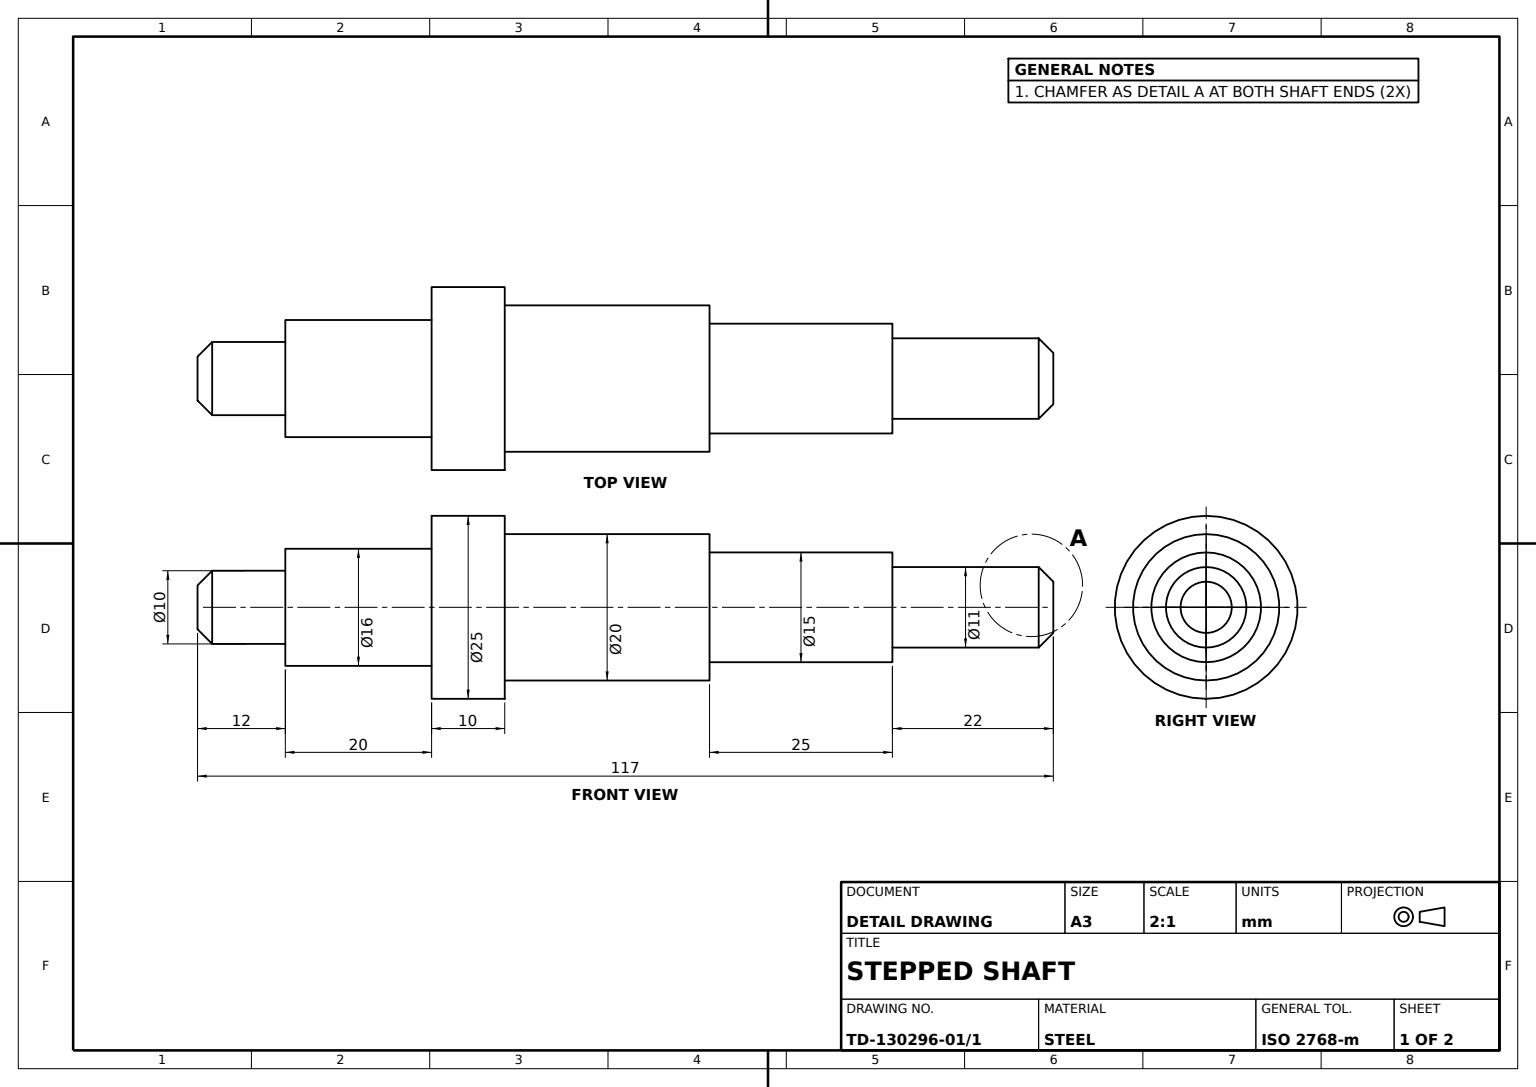
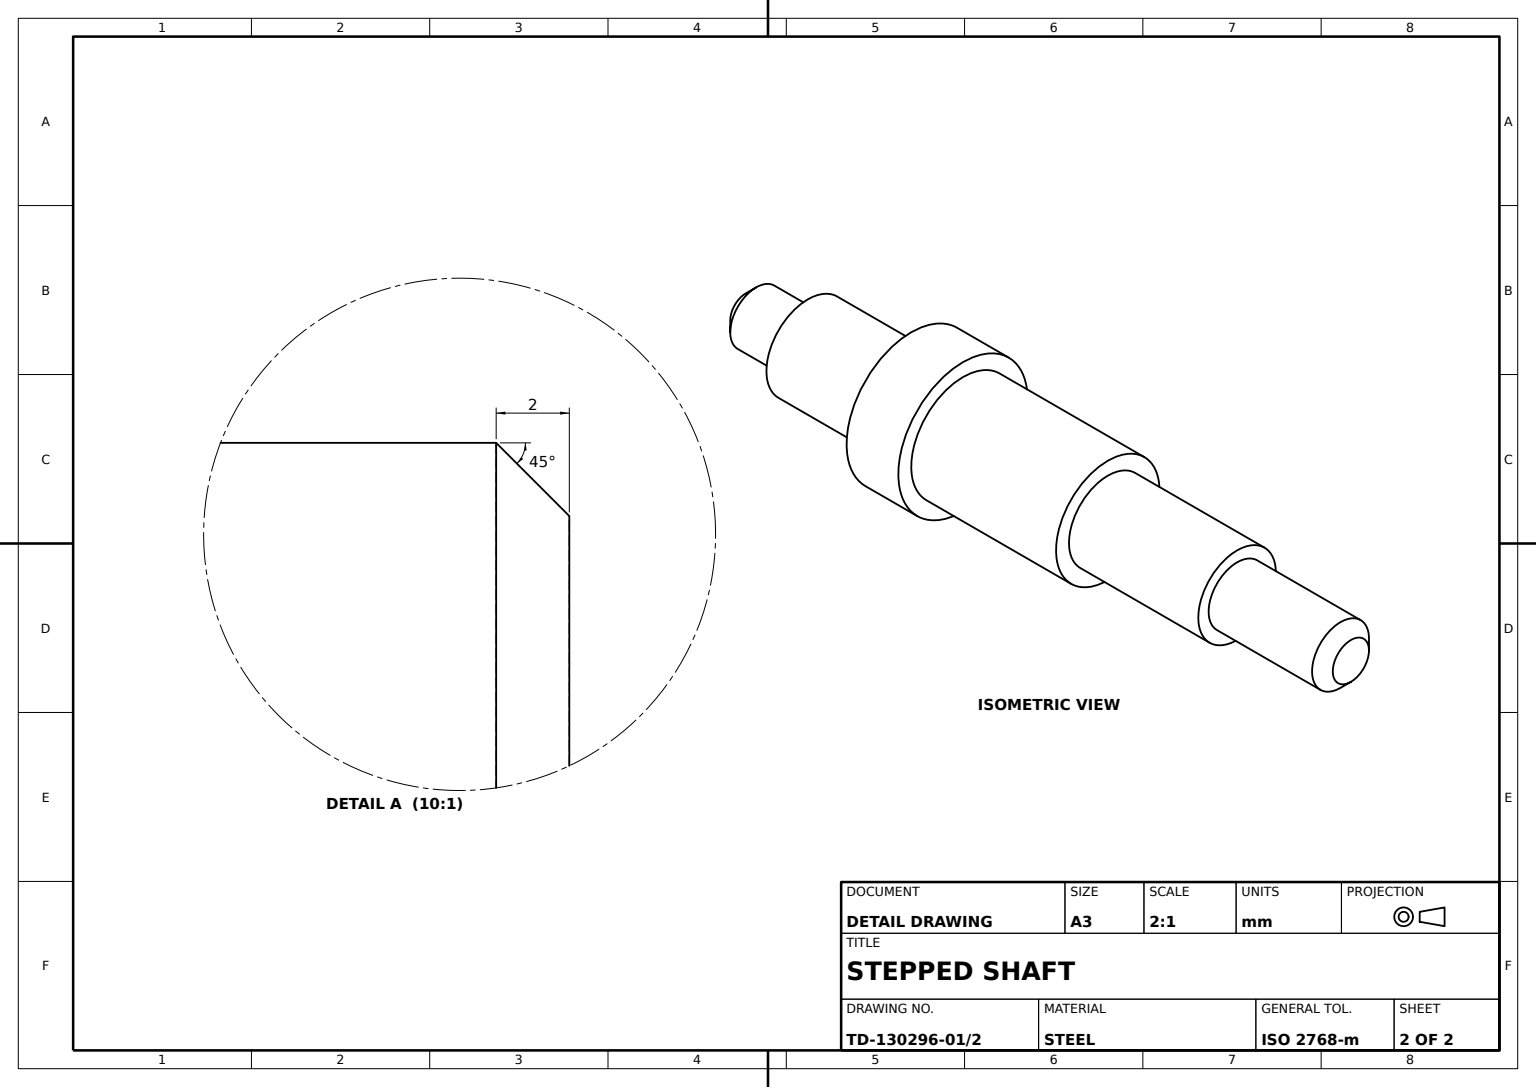
from build123d import *

# Parameters (mm, degrees)
EDGE_CHAMFER_2X45_SIZE = 2


with BuildPart() as part:
    # Shaft Profile Sketch → Stepped Shaft Revolve (revolve)
    with BuildSketch(Plane.XY):
        Polygon((-58.5, 0), (-58.5, -5), (-46.5, -5), (-46.5, -8), (-26.5, -8), (-26.5, -12.5), (-16.5, -12.5), (-16.5, -10), (11.5, -10), (11.5, -7.5), (36.5, -7.5), (36.5, -5.5), (58.5, -5.5), (58.5, 0), align=None)
    revolve(axis=Axis((-58.5, 0, 0), (1, 0, 0)))

    # Edge Chamfer 2x45°
    edge_chamfer_2x45_edges = [part.edges().sort_by_distance(p)[0] for p in [
        (58.5, 5.5, 0),
        (-58.5, 5, 0),
    ]]
    chamfer(edge_chamfer_2x45_edges, length=EDGE_CHAMFER_2X45_SIZE)


solid = part.part
